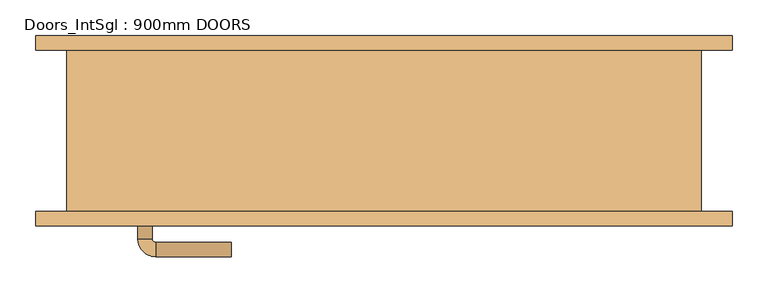
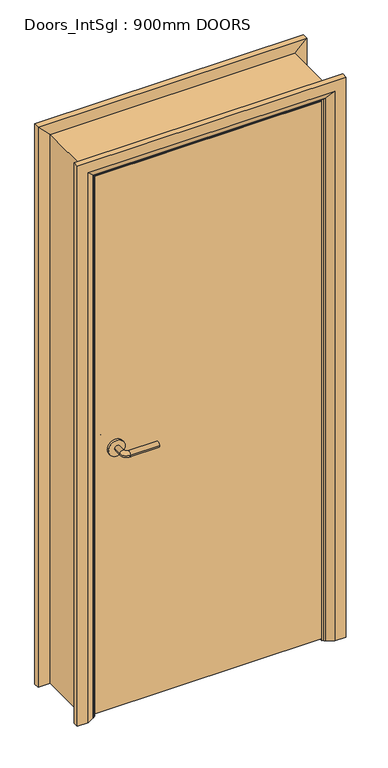
"""IFC4 building model written with IfcOpenShell, lengths in millimetres: door geometry, Doors_IntSgl : 900mm DOORS."""

from ifc_helpers import new_model, si_unit, point, frame, frame_2d, origin, place, context, project, spatial, polyline, circle_curve, ellipse_curve, trimmed, segment, composite_curve, outline, extrude, faceted_brep, source, transform, mapped, element, save
from ifc_brep_helpers import plane_surface, cylinder_surface, revolved_surface, advanced_brep


def doors_intsgl_900mm_doors_d21b38ee(model_context):
    return source(origin(), model_context, "Body", "SolidModel", [
        advanced_brep(
        [(-343.0, -66.5, 1000.0), (-323.0, -66.5, 1000.0), (-343.0, -36.5, 1000.0), (-323.0, -36.5, 1000.0), (-318.0, -31.5, 1000.0), (-318.0, -11.5, 1000.0), (-213.0, -11.5, 1000.0), (-213.0, -31.5, 1000.0)],
        [
            (0, 1, circle_curve(frame((-333.0, -66.5, 1000.0), z_axis=(0.0, -1.0, 0.0), x_axis=(1.0, 0.0, 0.0)), 10.0)),
            (1, 0, circle_curve(frame((-333.0, -66.5, 1000.0), z_axis=(0.0, -1.0, 0.0), x_axis=(1.0, 0.0, 0.0)), 10.0)),
            (0, 2),
            (2, 3, circle_curve(frame((-333.0, -36.5, 1000.0), z_axis=(0.0, -1.0, 0.0), x_axis=(1.0, 0.0, 0.0)), 10.0)),
            (3, 1),
            (3, 2, circle_curve(frame((-333.0, -36.5, 1000.0), z_axis=(0.0, -1.0, 0.0), x_axis=(1.0, 0.0, 0.0)), 10.0)),
            (4, 3, circle_curve(frame((-318.0, -36.5, 1000.0), z_axis=(0.0, 0.0, 1.0), x_axis=(-1.0, 0.0, 0.0)), 5.0)),
            (2, 5, circle_curve(frame((-318.0, -36.5, 1000.0), z_axis=(0.0, 0.0, -1.0), x_axis=(-1.0, 0.0, 0.0)), 25.0)),
            (5, 4, circle_curve(frame((-318.0, -21.5, 1000.0), z_axis=(-1.0, 0.0, 0.0), x_axis=(0.0, -1.0, 0.0)), 10.0)),
            (4, 5, circle_curve(frame((-318.0, -21.5, 1000.0), z_axis=(-1.0, 0.0, 0.0), x_axis=(0.0, -1.0, 0.0)), 10.0)),
            (6, 7, circle_curve(frame((-213.0, -21.5, 1000.0), z_axis=(1.0, 0.0, 0.0), x_axis=(0.0, -1.0, 0.0)), 10.0)),
            (7, 6, circle_curve(frame((-213.0, -21.5, 1000.0), z_axis=(1.0, 0.0, 0.0), x_axis=(0.0, -1.0, 0.0)), 10.0)),
            (5, 6),
            (7, 4),
        ],
        [
            plane_surface(frame((-333.0, -66.5, 1000.0), z_axis=(0.0, -1.0, 0.0), x_axis=(0.0, 0.0, 1.0))),
            cylinder_surface(frame((-333.0, -66.5, 1000.0), z_axis=(0.0, -1.0, 0.0), x_axis=(1.0, 0.0, 0.0)), 10.0),
            revolved_surface(trimmed(ellipse_curve(frame((-333.0, -36.5, 1000.0), z_axis=(0.0, -1.0, 0.0), x_axis=(1.0, 0.0, 0.0)), 10.0, 10.0), [point((-343.0, -36.5, 1000.0))], [point((-323.0, -36.5, 1000.0))], True, "CARTESIAN"), (-318.0, -36.5, 1000.0), (0.0, 0.0, -1.0)),
            revolved_surface(trimmed(ellipse_curve(frame((-333.0, -36.5, 1000.0), z_axis=(0.0, -1.0, 0.0), x_axis=(1.0, 0.0, 0.0)), 10.0, 10.0), [point((-323.0, -36.5, 1000.0))], [point((-343.0, -36.5, 1000.0))], True, "CARTESIAN"), (-318.0, -36.5, 1000.0), (0.0, 0.0, -1.0)),
            plane_surface(frame((-213.0, -21.5, 1000.0), z_axis=(1.0, 0.0, 0.0), x_axis=(0.0, 0.0, 1.0))),
            cylinder_surface(frame((-318.0, -21.5, 1000.0), z_axis=(-1.0, 0.0, 0.0), x_axis=(0.0, -1.0, 0.0)), 10.0),
        ],
        [
            (0, [[1, 2]]),
            (1, [[-1, 3, 4, 5]]),
            (1, [[-2, -5, 6, -3]]),
            (2, [[7, -4, 8, 9]]),
            (3, [[-8, -6, -7, 10]]),
            (4, [[11, 12]]),
            (5, [[-9, 13, -12, 14]]),
            (5, [[-10, -14, -11, -13]]),
        ],
    ),
        extrude(outline(composite_curve([segment(trimmed(circle_curve(frame_2d((1000.0, -335.5)), 30.0), [point((1000.0, -365.5))], [point((1000.0, -305.5))], False, "CARTESIAN"), True, "CONTINUOUS"), segment(trimmed(circle_curve(frame_2d((1000.0, -335.5)), 30.0), [point((1000.0, -305.5))], [point((1000.0, -365.5))], False, "CARTESIAN"), True, "CONTINUOUS")], self_intersect=False)), frame((0.0, -74.5, 0.0), z_axis=(0.0, 1.0, 0.0), x_axis=(0.0, 0.0, 1.0)), (0.0, 0.0, 1.0), 8.0),
        advanced_brep(
        [(-343.0, -120.5, 1000.0), (-323.0, -120.5, 1000.0), (-323.0, -150.5, 1000.0), (-343.0, -150.5, 1000.0), (-318.0, -155.5, 1000.0), (-318.0, -175.5, 1000.0), (-213.0, -175.5, 1000.0), (-213.0, -155.5, 1000.0)],
        [
            (0, 1, circle_curve(frame((-333.0, -120.5, 1000.0), z_axis=(0.0, 1.0, 0.0), x_axis=(1.0, 0.0, 0.0)), 10.0)),
            (1, 0, circle_curve(frame((-333.0, -120.5, 1000.0), z_axis=(0.0, 1.0, 0.0), x_axis=(1.0, 0.0, 0.0)), 10.0)),
            (1, 2),
            (2, 3, circle_curve(frame((-333.0, -150.5, 1000.0), z_axis=(0.0, 1.0, 0.0), x_axis=(1.0, 0.0, 0.0)), 10.0)),
            (3, 0),
            (3, 2, circle_curve(frame((-333.0, -150.5, 1000.0), z_axis=(0.0, 1.0, 0.0), x_axis=(1.0, 0.0, 0.0)), 10.0)),
            (4, 5, circle_curve(frame((-318.0, -165.5, 1000.0), z_axis=(-1.0, 0.0, 0.0), x_axis=(0.0, 1.0, 0.0)), 10.0)),
            (5, 3, circle_curve(frame((-318.0, -150.5, 1000.0), z_axis=(0.0, 0.0, -1.0), x_axis=(-1.0, 0.0, 0.0)), 25.0)),
            (2, 4, circle_curve(frame((-318.0, -150.5, 1000.0), z_axis=(0.0, 0.0, 1.0), x_axis=(-1.0, 0.0, 0.0)), 5.0)),
            (5, 4, circle_curve(frame((-318.0, -165.5, 1000.0), z_axis=(-1.0, 0.0, 0.0), x_axis=(0.0, 1.0, 0.0)), 10.0)),
            (6, 7, circle_curve(frame((-213.0, -165.5, 1000.0), z_axis=(1.0, 0.0, 0.0), x_axis=(0.0, 1.0, 0.0)), 10.0)),
            (7, 6, circle_curve(frame((-213.0, -165.5, 1000.0), z_axis=(1.0, 0.0, 0.0), x_axis=(0.0, 1.0, 0.0)), 10.0)),
            (4, 7),
            (6, 5),
        ],
        [
            plane_surface(frame((-333.0, -120.5, 1000.0), z_axis=(0.0, 1.0, 0.0), x_axis=(0.0, 0.0, 1.0))),
            cylinder_surface(frame((-333.0, -120.5, 1000.0), z_axis=(0.0, 1.0, 0.0), x_axis=(1.0, 0.0, 0.0)), 10.0),
            revolved_surface(trimmed(ellipse_curve(frame((-333.0, -150.5, 1000.0), z_axis=(0.0, -1.0, 0.0), x_axis=(1.0, 0.0, 0.0)), 10.0, 10.0), [point((-343.0, -150.5, 1000.0))], [point((-323.0, -150.5, 1000.0))], True, "CARTESIAN"), (-318.0, -150.5, 1000.0), (0.0, 0.0, -1.0)),
            revolved_surface(trimmed(ellipse_curve(frame((-333.0, -150.5, 1000.0), z_axis=(0.0, -1.0, 0.0), x_axis=(1.0, 0.0, 0.0)), 10.0, 10.0), [point((-323.0, -150.5, 1000.0))], [point((-343.0, -150.5, 1000.0))], True, "CARTESIAN"), (-318.0, -150.5, 1000.0), (0.0, 0.0, -1.0)),
            plane_surface(frame((-213.0, -165.5, 1000.0), z_axis=(1.0, 0.0, 0.0), x_axis=(0.0, 0.0, 1.0))),
            cylinder_surface(frame((-318.0, -165.5, 1000.0), z_axis=(-1.0, 0.0, 0.0), x_axis=(0.0, 1.0, 0.0)), 10.0),
        ],
        [
            (0, [[1, 2]]),
            (1, [[3, 4, 5, -2]]),
            (1, [[-5, 6, -3, -1]]),
            (2, [[7, 8, -4, 9]]),
            (3, [[10, -9, -6, -8]]),
            (4, [[11, 12]]),
            (5, [[13, -11, 14, -7]]),
            (5, [[-14, -12, -13, -10]]),
        ],
    ),
        extrude(outline(composite_curve([segment(trimmed(circle_curve(frame_2d((1000.0, -335.5)), 30.0), [point((1000.0, -365.5))], [point((1000.0, -305.5))], False, "CARTESIAN"), True, "CONTINUOUS"), segment(trimmed(circle_curve(frame_2d((1000.0, -335.5)), 30.0), [point((1000.0, -305.5))], [point((1000.0, -365.5))], False, "CARTESIAN"), True, "CONTINUOUS")], self_intersect=False)), frame((0.0, -120.5, 0.0), z_axis=(0.0, 1.0, 0.0), x_axis=(0.0, 0.0, 1.0)), (0.0, 0.0, 1.0), 8.0),
        extrude(outline(polyline([(408.0, -74.5), (408.0, -112.5), (-408.0, -112.5), (-408.0, -74.5), (408.0, -74.5)])), frame((0.0, 0.0, 8.0), z_axis=(0.0, 0.0, 1.0), x_axis=(1.0, 0.0, 0.0)), (0.0, 0.0, 1.0), 2050.0),
        faceted_brep([(-410.0, -112.5, 0.0), (-442.0, -112.5, 0.0), (-442.0, 112.5, 0.0), (-410.0, 112.5, 0.0), (-410.0, 112.5, 2060.0), (-410.0, -112.5, 2060.0), (-442.0, 112.5, 2092.0), (-442.0, -112.5, 2092.0), (410.0, -112.5, 0.0), (410.0, 112.5, 0.0), (442.0, 112.5, 0.0), (442.0, -112.5, 0.0), (410.0, -112.5, 2060.0), (442.0, -112.5, 2092.0), (442.0, 112.5, 2092.0), (410.0, 112.5, 2060.0)], [[[0, 1, 2, 3]], [[3, 4, 5, 0]], [[2, 6, 4, 3]], [[1, 7, 6, 2]], [[0, 5, 7, 1]], [[8, 9, 10, 11]], [[12, 8, 11, 13]], [[13, 11, 10, 14]], [[14, 10, 9, 15]], [[15, 9, 8, 12]], [[4, 15, 12, 5]], [[6, 14, 15, 4]], [[7, 13, 14, 6]], [[5, 12, 13, 7]]]),
        advanced_brep(
        [(-485.0, 132.5, 0.0), (-445.0, 132.5, 0.0), (-419.0, 118.5, 0.0), (-415.0, 112.5, 0.0), (-485.0, 112.5, 0.0), (-485.0, 112.5, 2135.0), (-485.0, 132.5, 2135.0), (-415.0, 112.5, 2065.0), (-419.0, 118.5, 2069.0), (-445.0, 132.5, 2095.0), (485.0, 132.5, 0.0), (485.0, 112.5, 0.0), (415.0, 112.5, 0.0), (419.0, 118.5, 0.0), (445.0, 132.5, 0.0), (485.0, 132.5, 2135.0), (445.0, 132.5, 2095.0), (419.0, 118.5, 2069.0), (415.0, 112.5, 2065.0), (485.0, 112.5, 2135.0)],
        [
            (0, 1),
            (1, 2),
            (2, 3, circle_curve(frame((-423.0, 111.5, 0.0), z_axis=(0.0, 0.0, -1.0), x_axis=(-1.0, 0.0, 0.0)), 8.0622577)),
            (3, 4),
            (4, 0),
            (4, 5),
            (5, 6),
            (6, 0),
            (3, 7),
            (7, 5),
            (2, 8),
            (8, 7, ellipse_curve(frame((-423.0, 111.5, 2073.0), z_axis=(-0.7071067811865475, 0.0, -0.7071067811865475), x_axis=(0.7071067811865474, 0.0, -0.7071067811865476)), 11.4017543, 8.0622577)),
            (1, 9),
            (9, 8),
            (6, 9),
            (10, 11),
            (11, 12),
            (12, 13, circle_curve(frame((423.0, 111.5, 0.0), z_axis=(0.0, 0.0, -1.0), x_axis=(1.0, 0.0, 0.0)), 8.0622577)),
            (13, 14),
            (14, 10),
            (15, 10),
            (14, 16),
            (16, 15),
            (13, 17),
            (17, 16),
            (12, 18),
            (18, 17, ellipse_curve(frame((423.0, 111.5, 2073.0), z_axis=(0.7071067811865475, 0.0, -0.7071067811865475), x_axis=(0.7071067811865474, 0.0, 0.7071067811865476)), 11.4017543, 8.0622577)),
            (11, 19),
            (19, 18),
            (15, 19),
            (5, 19),
            (15, 6),
            (7, 18),
            (8, 17),
            (9, 16),
        ],
        [
            plane_surface(frame((-415.0, 185.3010989, 0.0), z_axis=(0.0, 0.0, -1.0), x_axis=(1.0, 0.0, 0.0))),
            plane_surface(frame((-485.0, 132.5, 0.0), z_axis=(-1.0, 0.0, 0.0), x_axis=(0.0, 0.0, 1.0))),
            plane_surface(frame((-485.0, 112.5, 0.0), z_axis=(0.0, -1.0, 0.0), x_axis=(0.0, 0.0, 1.0))),
            cylinder_surface(frame((-423.0, 111.5, 0.0), z_axis=(0.0, 0.0, -1.0), x_axis=(-1.0, 0.0, 0.0)), 8.0622577),
            plane_surface(frame((-419.0, 118.5, 0.0), z_axis=(0.4740998230350183, 0.8804710999221749, 0.0), x_axis=(0.0, 0.0, 1.0))),
            plane_surface(frame((-445.0, 132.5, 0.0), z_axis=(0.0, 1.0, 0.0), x_axis=(0.0, 0.0, 1.0))),
            plane_surface(frame((415.0, 185.3010989, 0.0), z_axis=(0.0, 0.0, -1.0), x_axis=(-1.0, 0.0, 0.0))),
            plane_surface(frame((445.0, 132.5, 2095.0), z_axis=(0.0, 1.0, 0.0), x_axis=(0.0, 0.0, -1.0))),
            plane_surface(frame((419.0, 118.5, 2069.0), z_axis=(-0.4740998230350183, 0.8804710999221749, 0.0), x_axis=(0.0, 0.0, -1.0))),
            cylinder_surface(frame((423.0, 111.5, 2065.0), z_axis=(0.0, 0.0, 1.0), x_axis=(1.0, 0.0, 0.0)), 8.0622577),
            plane_surface(frame((485.0, 112.5, 2135.0), z_axis=(0.0, -1.0, 0.0), x_axis=(0.0, 0.0, -1.0))),
            plane_surface(frame((485.0, 132.5, 2135.0), z_axis=(1.0, 0.0, 0.0), x_axis=(0.0, 0.0, -1.0))),
            plane_surface(frame((-485.0, 132.5, 2135.0), z_axis=(0.0, 0.0, 1.0), x_axis=(1.0, 0.0, 0.0))),
            plane_surface(frame((-485.0, 112.5, 2135.0), z_axis=(0.0, -1.0, 0.0), x_axis=(1.0, 0.0, 0.0))),
            cylinder_surface(frame((-415.0, 111.5, 2073.0), z_axis=(-1.0, 0.0, 0.0), x_axis=(0.0, 0.0, 1.0)), 8.0622577),
            plane_surface(frame((-419.0, 118.5, 2069.0), z_axis=(0.0, 0.8804710999221749, -0.4740998230350183), x_axis=(1.0, 0.0, 0.0))),
            plane_surface(frame((-445.0, 132.5, 2095.0), z_axis=(0.0, 1.0, 0.0), x_axis=(1.0, 0.0, 0.0))),
        ],
        [
            (0, [[1, 2, 3, 4, 5]]),
            (1, [[6, 7, 8, -5]]),
            (2, [[9, 10, -6, -4]]),
            (3, [[11, 12, -9, -3]]),
            (4, [[13, 14, -11, -2]]),
            (5, [[-8, 15, -13, -1]]),
            (6, [[16, 17, 18, 19, 20]]),
            (7, [[21, -20, 22, 23]]),
            (8, [[-22, -19, 24, 25]]),
            (9, [[-24, -18, 26, 27]]),
            (10, [[-26, -17, 28, 29]]),
            (11, [[-28, -16, -21, 30]]),
            (12, [[31, -30, 32, -7]]),
            (13, [[33, -29, -31, -10]]),
            (14, [[34, -27, -33, -12]]),
            (15, [[35, -25, -34, -14]]),
            (16, [[-32, -23, -35, -15]]),
        ],
    ),
        extrude(outline(polyline([(0.0, -391.0), (2041.0, -391.0), (2041.0, 391.0), (0.0, 391.0), (0.0, 410.0), (2060.0, 410.0), (2060.0, -410.0), (0.0, -410.0), (0.0, -391.0)])), frame((0.0, -72.5, 0.0), z_axis=(0.0, 1.0, 0.0), x_axis=(0.0, 0.0, 1.0)), (0.0, 0.0, 1.0), 32.0),
        advanced_brep(
        [(485.0, -132.5, 0.0), (445.0, -132.5, 0.0), (419.0, -118.5, 0.0), (415.0, -112.5, 0.0), (485.0, -112.5, 0.0), (485.0, -112.5, 2135.0), (485.0, -132.5, 2135.0), (415.0, -112.5, 2065.0), (-415.0, -112.5, 2065.0), (-415.0, -112.5, 0.0), (-485.0, -112.5, 0.0), (-485.0, -112.5, 2135.0), (419.0, -118.5, 2069.0), (445.0, -132.5, 2095.0), (-485.0, -132.5, 2135.0), (-485.0, -132.5, 0.0), (-445.0, -132.5, 0.0), (-445.0, -132.5, 2095.0), (-419.0, -118.5, 0.0), (-419.0, -118.5, 2069.0)],
        [
            (0, 1),
            (1, 2),
            (2, 3, circle_curve(frame((423.0, -111.5, 0.0), z_axis=(0.0, 0.0, -1.0), x_axis=(1.0, 0.0, 0.0)), 8.0622577)),
            (3, 4),
            (4, 0),
            (4, 5),
            (5, 6),
            (6, 0),
            (3, 7),
            (7, 8),
            (8, 9),
            (9, 10),
            (10, 11),
            (11, 5),
            (2, 12),
            (12, 7, ellipse_curve(frame((423.0, -111.5, 2073.0), z_axis=(0.7071067811865475, 0.0, -0.7071067811865475), x_axis=(-0.7071067811865474, 0.0, -0.7071067811865476)), 11.4017543, 8.0622577)),
            (1, 13),
            (13, 12),
            (6, 14),
            (14, 15),
            (15, 16),
            (16, 17),
            (17, 13),
            (10, 15),
            (14, 11),
            (9, 18, circle_curve(frame((-423.0, -111.5, 0.0), z_axis=(0.0, 0.0, -1.0), x_axis=(-1.0, 0.0, 0.0)), 8.0622577)),
            (18, 16),
            (19, 18),
            (8, 19, ellipse_curve(frame((-423.0, -111.5, 2073.0), z_axis=(-0.7071067811865475, 0.0, -0.7071067811865475), x_axis=(-0.7071067811865474, 0.0, 0.7071067811865476)), 11.4017543, 8.0622577)),
            (19, 17),
            (12, 19),
        ],
        [
            plane_surface(frame((415.0, -112.5, 0.0), z_axis=(0.0, 0.0, -1.0), x_axis=(0.0, 1.0, 0.0))),
            plane_surface(frame((485.0, -132.5, 0.0), z_axis=(1.0, 0.0, 0.0), x_axis=(0.0, 0.0, 1.0))),
            plane_surface(frame((485.0, -112.5, 0.0), z_axis=(0.0, 1.0, 0.0), x_axis=(0.0, 0.0, 1.0))),
            cylinder_surface(frame((423.0, -111.5, 0.0), z_axis=(0.0, 0.0, -1.0), x_axis=(1.0, 0.0, 0.0)), 8.0622577),
            plane_surface(frame((419.0, -118.5, 0.0), z_axis=(-0.4740998230350126, -0.880471099922178, 0.0), x_axis=(0.0, 0.0, 1.0))),
            plane_surface(frame((445.0, -132.5, 0.0), z_axis=(0.0, -1.0, 0.0), x_axis=(0.0, 0.0, 1.0))),
            plane_surface(frame((-485.0, -132.5, 2135.0), z_axis=(-1.0, 0.0, 0.0), x_axis=(0.0, 0.0, -1.0))),
            plane_surface(frame((-415.0, -112.5, 0.0), z_axis=(0.0, 0.0, -1.0), x_axis=(0.0, 1.0, 0.0))),
            cylinder_surface(frame((-423.0, -111.5, 2065.0), z_axis=(0.0, 0.0, 1.0), x_axis=(-1.0, 0.0, 0.0)), 8.0622577),
            plane_surface(frame((-419.0, -118.5, 2069.0), z_axis=(0.47409982303501824, -0.8804710999221749, 0.0), x_axis=(0.0, 0.0, -1.0))),
            plane_surface(frame((485.0, -132.5, 2135.0), z_axis=(0.0, 0.0, 1.0), x_axis=(-1.0, 0.0, 0.0))),
            cylinder_surface(frame((415.0, -111.5, 2073.0), z_axis=(1.0, 0.0, 0.0), x_axis=(0.0, 0.0, 1.0)), 8.0622577),
            plane_surface(frame((419.0, -118.5, 2069.0), z_axis=(0.0, -0.8804710999221764, -0.4740998230350154), x_axis=(-1.0, 0.0, 0.0))),
        ],
        [
            (0, [[1, 2, 3, 4, 5]]),
            (1, [[6, 7, 8, -5]]),
            (2, [[9, 10, 11, 12, 13, 14, -6, -4]]),
            (3, [[15, 16, -9, -3]]),
            (4, [[17, 18, -15, -2]]),
            (5, [[-8, 19, 20, 21, 22, 23, -17, -1]]),
            (6, [[-13, 24, -20, 25]]),
            (7, [[-24, -12, 26, 27, -21]]),
            (8, [[28, -26, -11, 29]]),
            (9, [[-22, -27, -28, 30]]),
            (10, [[-14, -25, -19, -7]]),
            (11, [[31, -29, -10, -16]]),
            (12, [[-23, -30, -31, -18]]),
        ],
    ),
    ])


if __name__ == "__main__":
    model = new_model("IFC4")
    model_context = context("Model", 3, world=origin())
    ifc_project = project(units=[si_unit("LENGTHUNIT", "METRE", prefix="MILLI")], contexts=[model_context])
    site = spatial("IfcSite", under=ifc_project)
    building = spatial("IfcBuilding", under=site)
    placement = place(None, origin())
    doors_intsgl_900mm_doors_shape = doors_intsgl_900mm_doors_d21b38ee(model_context)
    element("IfcDoor", 1, ObjectType="Doors_IntSgl : 900mm DOORS", at=placement, inside=building, context=model_context, shape_type="MappedRepresentation", body=[
        mapped(doors_intsgl_900mm_doors_shape, transform((0.0, 0.0, 0.0), x_axis=(1.0, 0.0, 0.0), y_axis=(0.0, 1.0, 0.0), z_axis=(0.0, 0.0, 1.0))),
    ])
    save(model, "model.ifc")

# Revit data of these elements
# Type "Doors_IntSgl : 900mm DOORS"
#   Type Mark = "46"
#   Type Comments = "Internal Single"
#   Operation = "SingleSwingRight"
#   Manufacturer = "Revit"
#   Keynote = "L20"
#   Description = "Internal Single Door"
#   Analytic Construction = "Metal"
#   UnderCut = 8 mm
#   Tolerance = 2 mm
#   Thickness = 38 mm
#   Thermal Resistance (R) = 0.270117 (m²·K)/W
#   Structural Tolerance = 8 mm
#   StopDepth = 32 mm
#   Stop Thickness = 19 mm
#   Rough Width = 900 mm
#   Rough Height = 2100 mm
#   Height to Top Lock Rail = 1000 mm
#   Heat Transfer Coefficient (U) = 3.7021 W/(m²·K)
#   Handle Z Distance = 1000 mm
#   Handle X Distance = 75 mm
#   Frame Thickness = 32 mm
#   Door Panel Width = 816 mm
#   Door Panel Thickness = 38 mm
#   Door Panel Offset = 0 mm
#   Height = 2100 mm
#   Width = 900 mm
#   Door Panel Height = 2050 mm
#   Architrave Setback = 5 mm
#   Vis - Ironmongery = yes
#   Define Thermal Properties by = 1
#   Material Ironmongery = Door - Handle
#   Material Frame = Door - Frame/Mullion (1)
#   Material Door = Door - Panel
#   Material Architrave = Door - Architrave
#   Visual Light Transmittance = 0
#   Solar Heat Gain Coefficient = 0
#   Function = (empty or 0)
#   Wall Closure = (empty or 0)
# Element 1 (IfcDoor, "Doors_IntSgl : 900mm DOORS")
#   Materials on its faces: "Door - Architrave", "Door - Handle", "Door - Frame/Mullion (1)", "Door - Panel"
# Materials
#   "Door - Handle": colour RGB 0 0 0, transparency 0, Cost = 0
#   "Door - Frame/Mullion (1)": class "Wood", colour RGB 212 179 113, transparency 0, Keynote = "L20", Cost = 0
#   "Door - Panel": class "Wood", colour RGB 210 159 95, transparency 0, Cost = 0
#   "Door - Architrave": class "Wood", colour RGB 154 90 5, transparency 0, Keynote = "P20", Cost = 0
